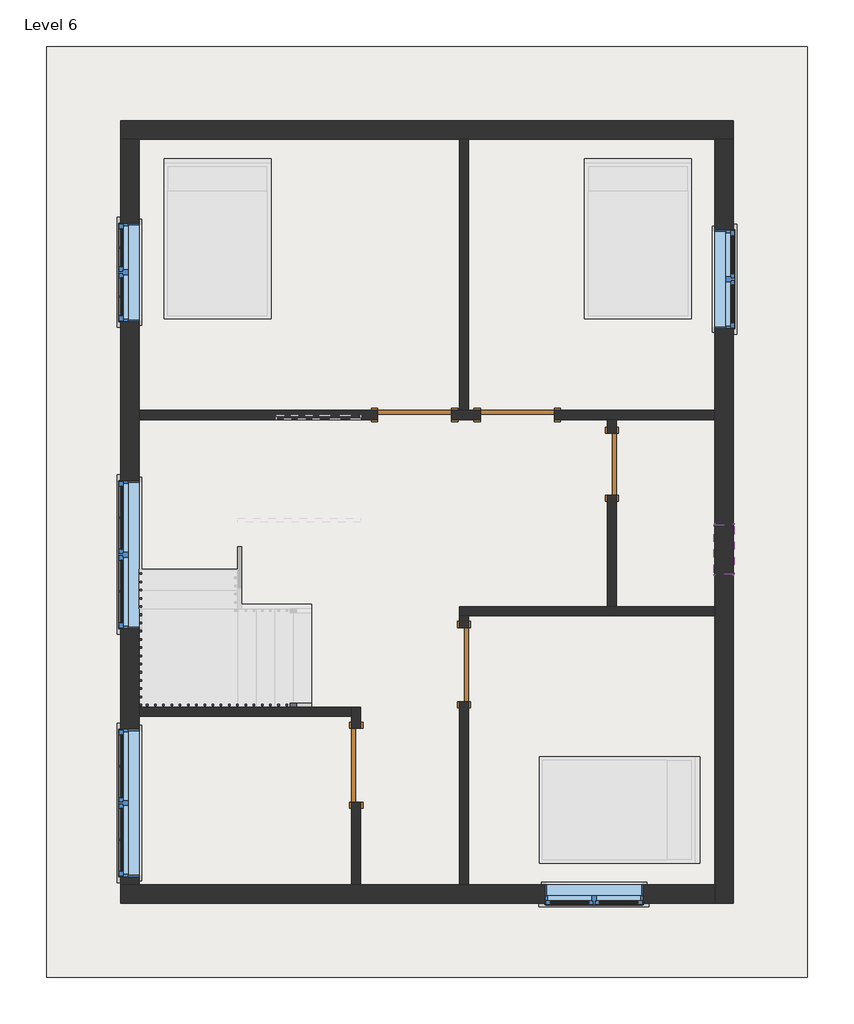
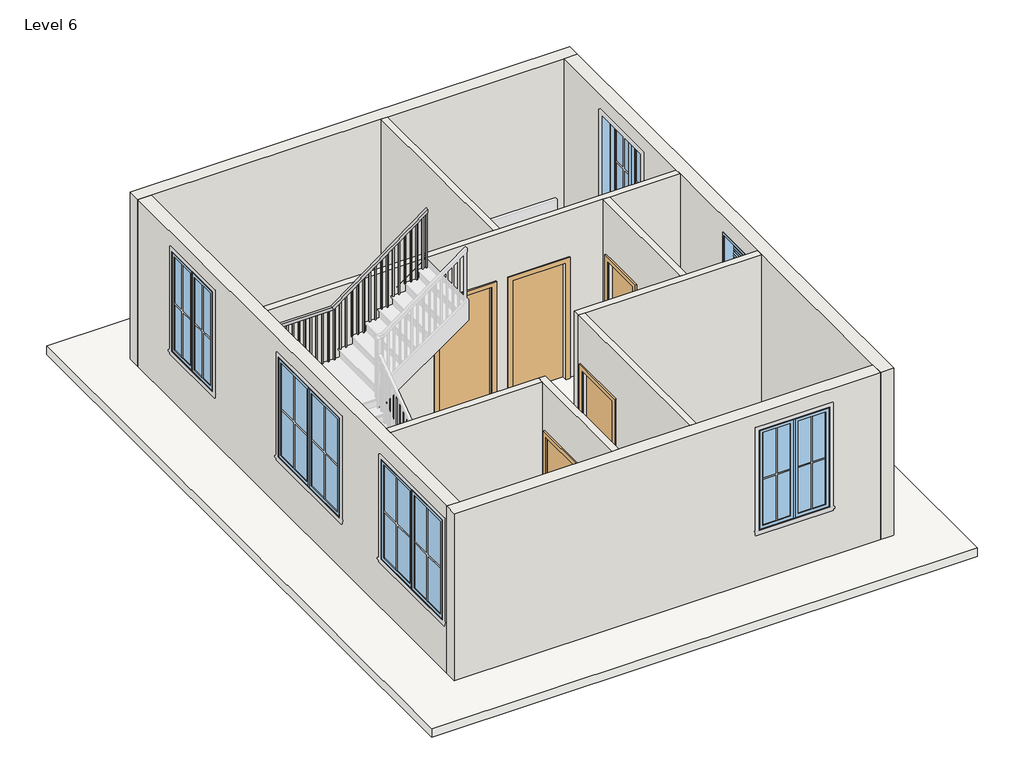
# One storey, part 1 of 2: 11 walls, 6 windows, 5 doors, 1 railing, 1 roof.
# Revit data of these elements (continued)
# Element 7 (IfcRoof, "Generic - 12\"") (continued)
#   built-in parameter 1001701 = -0.5 (stored number, unit not read)
#   built-in parameter 1001710 = 33615
#   Phase Created = New Construction
#   Materials on its faces: "Wood Planks", "Wood - Stained"
# Elements 8, 9, 10, 11, 12, 13, 14 (IfcWall, "WALL 4.5\"")
#   Top Offset = 0' - 0"
#   Base Offset = 0' - 0"
#   Unconnected Height = 10' - 0"
#   wall height = 10' - 0"
#   Phase Created = New Construction
#   Base Constraint = Level 6
#   Materials on its faces: "Default Wall"
# Elements 15, 16, 17, 18 (IfcWall, "WALL 9\"")
#   Top Offset = 0' - 0"
#   Base Offset = 0' - 0"
#   Unconnected Height = 10' - 0"
#   wall height = 10' - 0"
#   Phase Created = New Construction
#   Base Constraint = Level 6
#   Materials on its faces: "Default Wall", "Door - Frame"
# Element 19 (IfcWindow, "Window-Casement-Double : win 4'")
#   Mark = "33"
#   Window Inset = 0' - 0"
#   Interior Wall Closure = 0' - 2 1/4"
#   Frame Extension = 0' - 0 1/4"
#   Exterior Wall Closure = 0' - 1 1/4"
#   Interior Trim Visibility = yes
#   Exterior Trim Visibility = yes
#   Phase Created = New Construction
#   Materials on its faces: "Wood - Stained", "Glass", "Clad - White"
# Element 20 (IfcWindow, "Window-Casement-Double : win 4'")
#   Mark = "34"
#   Window Inset = 0' - 0"
#   Interior Wall Closure = 0' - 2 1/4"
#   Frame Extension = 0' - 0 1/4"
#   Exterior Wall Closure = 0' - 1 1/4"
#   Interior Trim Visibility = yes
#   Exterior Trim Visibility = yes
#   Phase Created = New Construction
#   Materials on its faces: "Wood - Stained", "Glass", "Clad - White"
# Element 21 (IfcWindow, "Window-Casement-Double : win 4'")
#   Mark = "35"
#   Window Inset = 0' - 0"
#   Interior Wall Closure = 0' - 2 1/4"
#   Frame Extension = 0' - 0 1/4"
#   Exterior Wall Closure = 0' - 1 1/4"
#   Interior Trim Visibility = yes
#   Exterior Trim Visibility = yes
#   Phase Created = New Construction
#   Materials on its faces: "Wood - Stained", "Glass", "Clad - White"
# Element 22 (IfcWindow, "Window-Casement-Double : win 6'")
#   Mark = "31"
#   Window Inset = 0' - 0"
#   Interior Wall Closure = 0' - 2 1/4"
#   Frame Extension = 0' - 0 1/4"
#   Exterior Wall Closure = 0' - 1 1/4"
#   Interior Trim Visibility = yes
#   Exterior Trim Visibility = yes
#   Phase Created = New Construction
#   Materials on its faces: "Wood - Stained", "Glass", "Clad - White"
# Element 23 (IfcWindow, "Window-Casement-Double : win 6'")
#   Mark = "32"
#   Window Inset = 0' - 0"
#   Interior Wall Closure = 0' - 2 1/4"
#   Frame Extension = 0' - 0 1/4"
#   Exterior Wall Closure = 0' - 1 1/4"
#   Interior Trim Visibility = yes
#   Exterior Trim Visibility = yes
#   Phase Created = New Construction
#   Materials on its faces: "Wood - Stained", "Glass", "Clad - White"
# Element 24 (IfcWindow, "Window-Louvers : 24\" x 24\"")
#   Mark = "36"
#   Blade Width = 1' - 10 1/2"
#   Phase Created = New Construction
#   Materials on its faces: "Birch"
# Materials
#   "Door - Panel": class "Wood", colour RGB 210 159 95, transparency 0, Cost = 0
#   "Door - Frame": colour RGB 118 70 51, transparency 0, Cost = 0
#   "Wood - Stained": class "Wood", colour RGB 224 178 126, transparency 0, Cost = 0
#   "Glass": class "Glass", colour RGB 0 128 192, transparency 0.75, Description = "Soda Lime Glass", Cost = 0
#   "Clad - White": class "Wood", colour RGB 242 242 238, transparency 0, Cost = 0
#   "Birch": class "Wood", colour RGB 224 178 126, transparency 0, Description = "Betula Alleghaniensis", Cost = 0
#   "Wood Planks": class "Wood", colour RGB 193 160 115, transparency 0, Description = "Physical material.", Cost = 0
#   "Default Wall": colour RGB 128 128 128, transparency 0, Cost = 0
